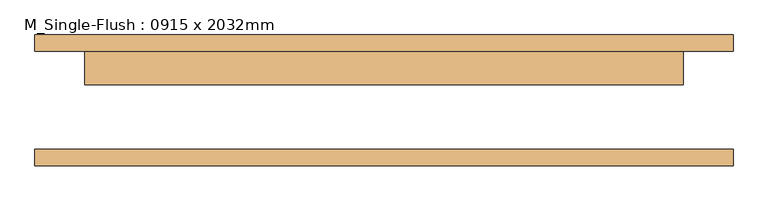
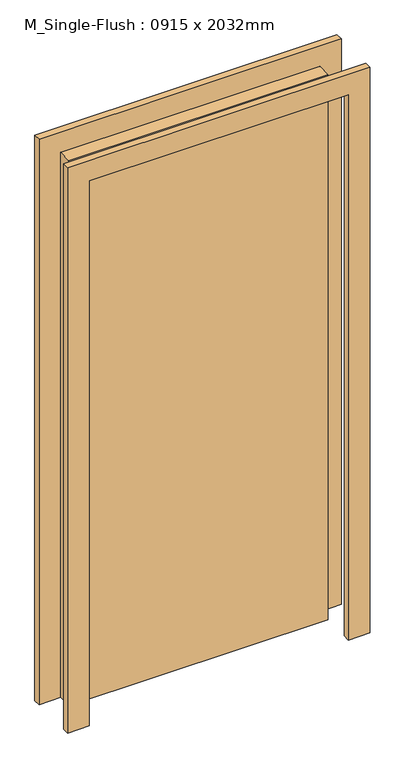
"""IFC4 building model written with IfcOpenShell, lengths in millimetres: door geometry, M_Single-Flush : 0915 x 2032mm."""

from ifc_helpers import new_model, si_unit, frame, origin, origin_with_axes, place, context, project, spatial, polyline, outline, extrude, source, transform, mapped, element, save


def m_single_flush_0915_x_2032mm_d0c19338(model_context):
    return source(origin(), model_context, "Body", "SweptSolid", [
        extrude(outline(polyline([(2108.0, -533.5), (0.0, -533.5), (0.0, -457.5), (2032.0, -457.5), (2032.0, 457.5), (0.0, 457.5), (0.0, 533.5), (2108.0, 533.5), (2108.0, -533.5)])), frame((0.0, 75.0, 0.0), z_axis=(0.0, 1.0, 0.0), x_axis=(0.0, 0.0, 1.0)), (0.0, 0.0, 1.0), 25.0),
        extrude(outline(polyline([(2108.0, 533.5), (2108.0, -533.5), (0.0, -533.5), (0.0, -457.5), (2032.0, -457.5), (2032.0, 457.5), (0.0, 457.5), (0.0, 533.5), (2108.0, 533.5)])), frame((0.0, -100.0, 0.0), z_axis=(0.0, 1.0, 0.0), x_axis=(0.0, 0.0, 1.0)), (0.0, 0.0, 1.0), 25.0),
        extrude(outline(polyline([(457.5, 24.0), (-457.5, 24.0), (-457.5, 75.0), (457.5, 75.0), (457.5, 24.0)])), origin_with_axes(), (0.0, 0.0, 1.0), 2032.0),
    ])


if __name__ == "__main__":
    model = new_model("IFC4")
    model_context = context("Model", 3, world=origin())
    ifc_project = project(units=[si_unit("LENGTHUNIT", "METRE", prefix="MILLI")], contexts=[model_context])
    site = spatial("IfcSite", under=ifc_project)
    building = spatial("IfcBuilding", under=site)
    placement = place(None, origin())
    m_single_flush_0915_x_2032mm_shape = m_single_flush_0915_x_2032mm_d0c19338(model_context)
    element("IfcDoor", 1, ObjectType="M_Single-Flush : 0915 x 2032mm", at=placement, inside=building, context=model_context, shape_type="MappedRepresentation", body=[
        mapped(m_single_flush_0915_x_2032mm_shape, transform((0.0, 0.0, 0.0), x_axis=(1.0, 0.0, 0.0), y_axis=(0.0, 1.0, 0.0), z_axis=(0.0, 0.0, 1.0))),
    ])
    save(model, "model.ifc")

# Revit data of these elements
# Type "M_Single-Flush : 0915 x 2032mm"
#   Type Mark = "20"
#   Thickness = 51 mm
#   Height = 2032 mm
#   Trim Projection Ext = 25 mm
#   Trim Projection Int = 25 mm
#   Trim Width = 76 mm
#   Width = 915 mm
#   Door Material = Door - Panel
#   Frame Material = Door - Frame
#   Function = (empty or 0)
#   Wall Closure = (empty or 0)
# Element 1 (IfcDoor, "M_Single-Flush : 0915 x 2032mm")
#   Materials on its faces: "Door - Frame", "Door - Panel"
# Materials
#   "Door - Panel": class "Wood", colour RGB 114 82 51, transparency 0
#   "Door - Frame": colour RGB 153 76 43, transparency 0
